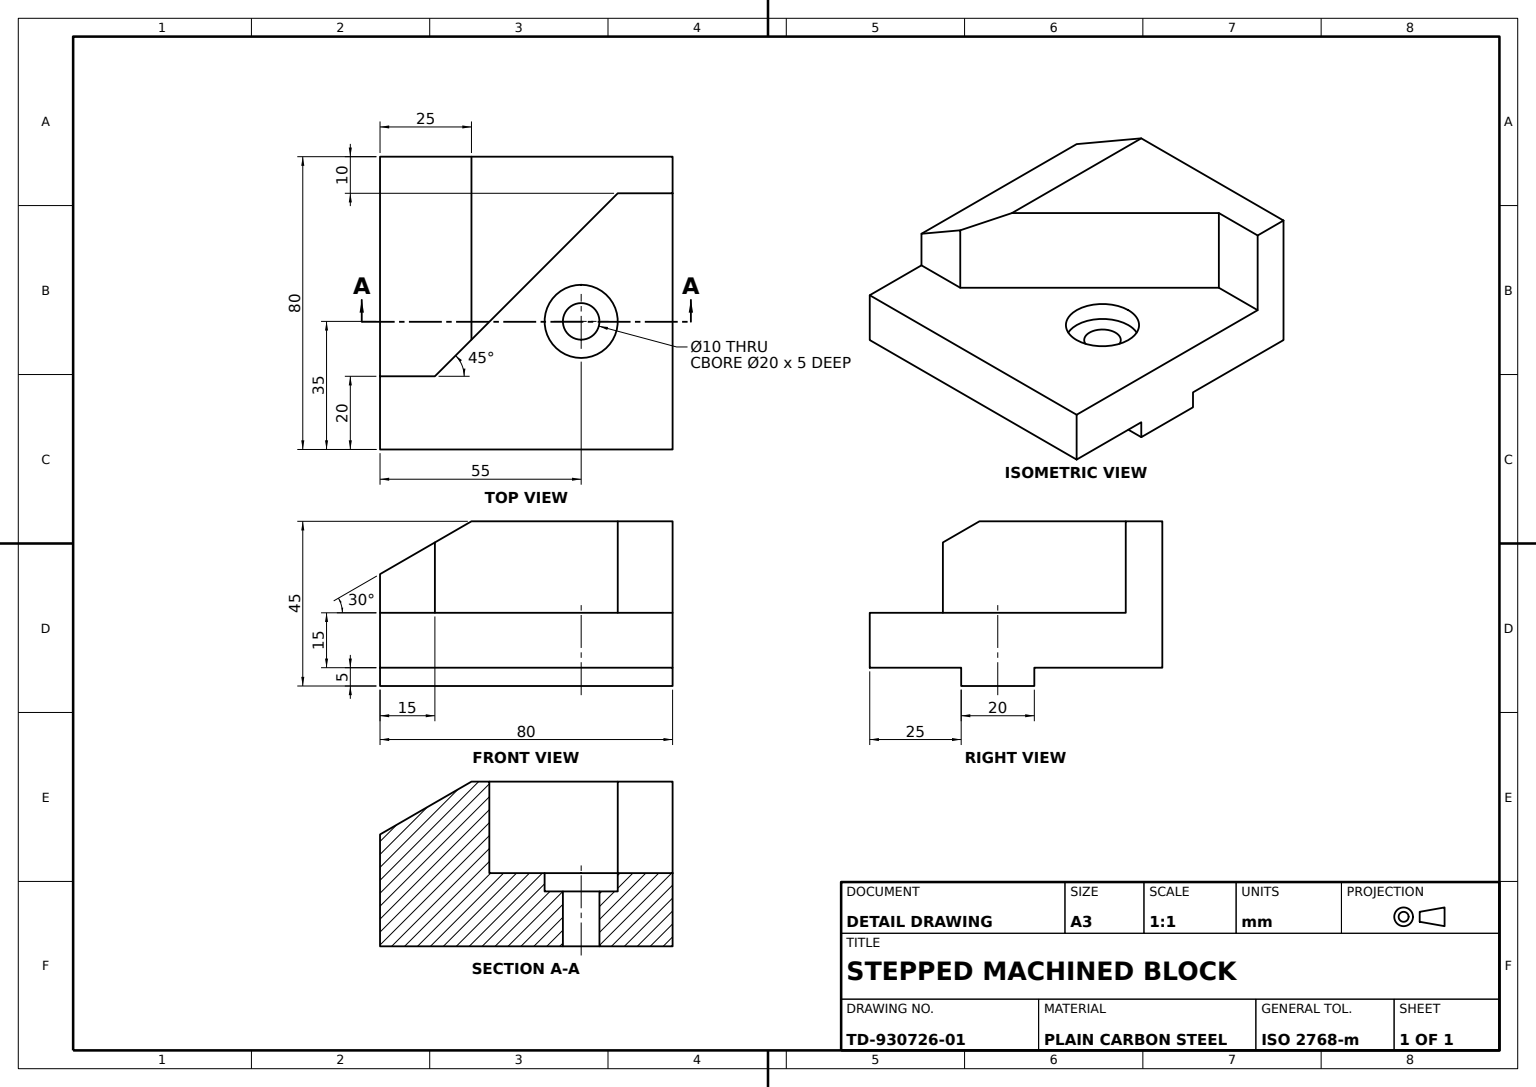
SolidWorks part; units mm, degrees
material "Plain Carbon Steel"
ref_plane "Front Plane" through (0, 0, 0) normal (0, 0, 1) x (1, 0, 0)
ref_plane "Top Plane" through (0, 0, 0) normal (0, 1, 0) x (1, 0, 0)
ref_plane "Right Plane" through (0, 0, 0) normal (1, 0, 0) x (0, 0, -1)
sketch "Base Plate Sketch 80x80" plane through (0, 0, 0) normal (0, 1, 0) x (1, 0, 0)
  line L1 (-40, 40) -> (40, 40)
  line L2 (-40, 40) -> (-40, -40)
  line L3 (-40, -40) -> (40, -40)
  line L4 (40, 40) -> (40, -40)
  line L5 (-40, 40) -> (40, -40) construction
  line L6 (-40, -40) -> (40, 40) construction
  point P0 (0, 0)
  dimension "D1" = 80
extrude "Base Plate 80x80x15" add sketch "Base Plate Sketch 80x80" along normal blind 15
sketch "Locating Key Sketch 20x25" plane through (0, 0, 0) normal (0, -1, 0) x (1, 0, 0)
  line L0 (-40, -40) -> (-40, 40) construction
  line L1 (-40, 15) -> (40, 15)
  line L2 (-40, 15) -> (-40, -5)
  line L3 (-40, -5) -> (40, -5)
  line L4 (40, 15) -> (40, -5)
  line L5 (40, 40) -> (40, -40) construction
  line L7 (-40, 40) -> (40, 40) construction
  dimension "D1" = 20
  dimension "D2" = 25
extrude "Locating Key 20x25x5" add sketch "Locating Key Sketch 20x25" along normal blind 5
sketch "Mounting Hole Sketch Ø10" plane through (0, 15, 0) normal (0, 1, 0) x (1, 0, 0)
  line L0 (-40, -40) -> (40, -40) construction
  line L1 (40, -40) -> (40, 40) construction
  circle A0 centre (15, -5) radius 5
  dimension "D1" = 10
  dimension "D2" = 35
  dimension "D3" = 25
extrude "Mounting Hole Ø10" cut sketch "Mounting Hole Sketch Ø10" against normal blind 60
sketch "Counterbore Sketch Ø20" plane through (0, 15, 0) normal (0, 1, 0) x (1, 0, 0)
  circle A0 centre (15, -5) radius 10
  dimension "D1" = 20
extrude "Counterbore Ø20x5" cut sketch "Counterbore Sketch Ø20" against normal blind 5
sketch "Stop Block Profile Sketch" plane through (0, 15, 0) normal (0, 1, 0) x (1, 0, 0)
  line L0 (40, 40) -> (40, 30)
  line L1 (40, -40) -> (40, 40) construction
  line L2 (40, 30) -> (25, 30)
  line L3 (40, 40) -> (-40, 40)
  line L4 (-40, 40) -> (-40, -20)
  line L5 (-40, 40) -> (-40, -40) construction
  line L6 (-40, -20) -> (-25, -20)
  line L7 (-25, -20) -> (25, 30)
  dimension "D1" = 10
  dimension "D2" = 15
  dimension "D3" = 60
  dimension "D4" = 15
extrude "Stop Block 25 High" add sketch "Stop Block Profile Sketch" along normal blind 25
sketch "V-Stop Angle Sketch 30deg" plane through (0, 0, -40) normal (0, 0, -1) x (-1, 0, 0)
  line L0 (40, 25.5662) -> (15, 40)
  line L1 (40, 40) -> (40, 0) construction
  line L2 (-40, 40) -> (40, 40) construction
  line L4 (40, 25.5662) -> (40, 40)
  line L5 (40, 40) -> (15, 40)
  dimension "D1" = 25
  dimension "D2" = 30
extrude "V-Stop Angled Face Cut 30deg" cut sketch "V-Stop Angle Sketch 30deg" against normal blind 100
